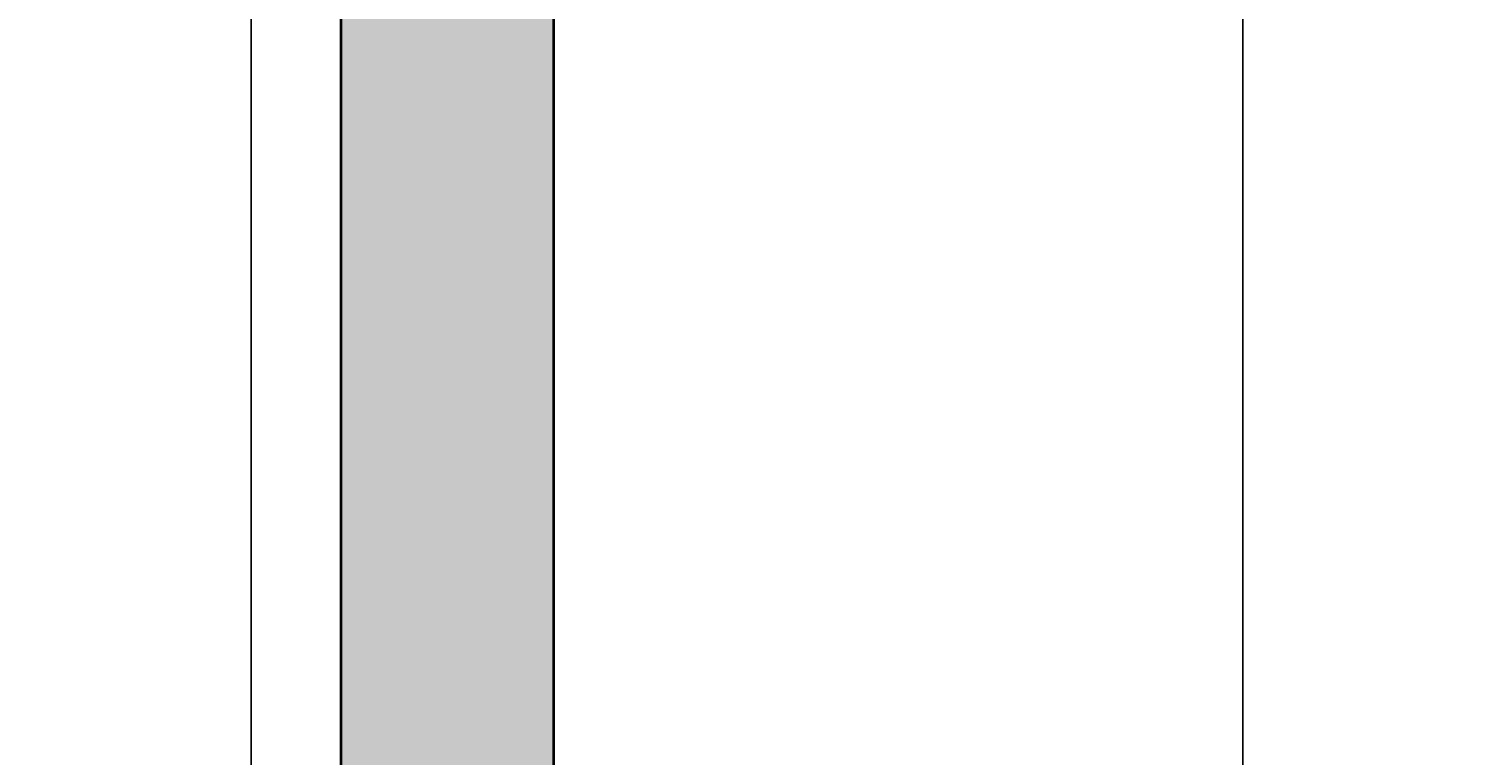
# Model space of a CAD drawing. Units: inches. Extents: x 1998 to 2588, y 1139 to 1977.
# Tile 131 of 134: x 2489 to 2550, y 1667 to 1698. Entities that reach past the tile are written whole.
import ezdxf

# ---------------------------------------------------------------- set-up
doc = ezdxf.new("R2010")
doc.units = ezdxf.units.IN
for name, color, linetype, lineweight in [('A-ANNO-DIMS', 2, 'Continuous', 18), ('A-WALL-PATT', 252, 'Continuous', 13), ('WALL', 200, 'Continuous', 35)]:
    doc.layers.add(name, color=color, linetype=linetype, lineweight=lineweight)
doc.styles.get("Standard").update_dxf_attribs({"font": 'arial.ttf'})
doc.dimstyles.get("Standard").update_dxf_attribs({"dimtxt": 0.18, "dimasz": 0.18, "dimexe": 0.18, "dimexo": 0.0625, "dimgap": 0.09, "dimtad": 0, "dimtih": 1, "dimtoh": 1, "dimdec": 4, "dimzin": 0, "dimdsep": 46, "dimtxsty": 'Standard', "dimcen": 0.09, "dimadec": 0, "dimazin": 0, "dimtfac": 1, "dimtdec": 4, "dimtofl": 0, "dimtmove": 0, "dimatfit": 3, "dimfxl": 1, "dimtolj": 1, "dimtzin": 0, "dimarcsym": 0})

# ---------------------------------------------------------------- blocks, each defined once
blk = doc.blocks.new('*D24')
at = {"layer": 'A-ANNO-DIMS', "color": 0, "lineweight": -2, "transparency": 16777216}
for p, q in [((2398.535, 1911.232), (2588.309, 1911.232)), ((2588.129, 1911.052), (2588.129, 1570.164)), ((2588.129, 1228.912), (2588.129, 1569.8)), ((2527.535, 1228.732), (2588.309, 1228.732))]:
    blk.add_line(p, q, dxfattribs=at)
at = {"layer": 'A-ANNO-DIMS', "color": 0, "transparency": 16777216}
for points in [[(2588.099, 1911.052), (2588.159, 1911.052), (2588.129, 1911.232)], [(2588.099, 1228.912), (2588.159, 1228.912), (2588.129, 1228.732)]]:
    blk.add_solid(points, dxfattribs=at)
at = {"layer": 'Defpoints', "color": 0, "transparency": 16777216}
for p in [(2398.473, 1911.232), (2588.129, 1911.232), (2527.473, 1228.732)]:
    blk.add_point(p, dxfattribs=at)
at = {"layer": 'A-ANNO-DIMS', "color": 0, "transparency": 16777216, "insert": (2588.129, 1569.982), "char_height": 0.18, "attachment_point": 5}
blk.add_mtext('\\A1;682.5', dxfattribs=at)
blk = doc.blocks.new('*D31')
at = {"layer": 'A-ANNO-DIMS', "color": 0, "lineweight": -2, "transparency": 16777216}
for p, q in [((2498.179, 1636.795), (2498.179, 1977.362)), ((2498.359, 1977.182), (2518.957, 1977.182)), ((2539.999, 1977.182), (2519.4, 1977.182)), ((2540.179, 1636.795), (2540.179, 1977.362))]:
    blk.add_line(p, q, dxfattribs=at)
at = {"layer": 'A-ANNO-DIMS', "color": 0, "transparency": 16777216}
for points in [[(2498.359, 1977.212), (2498.359, 1977.152), (2498.179, 1977.182)], [(2539.999, 1977.212), (2539.999, 1977.152), (2540.179, 1977.182)]]:
    blk.add_solid(points, dxfattribs=at)
at = {"layer": 'Defpoints', "color": 0, "transparency": 16777216}
for p in [(2540.179, 1977.182), (2498.179, 1636.732), (2540.179, 1636.732)]:
    blk.add_point(p, dxfattribs=at)
at = {"layer": 'A-ANNO-DIMS', "color": 0, "transparency": 16777216, "insert": (2519.179, 1977.182), "char_height": 0.18, "attachment_point": 5}
blk.add_mtext('\\A1;42', dxfattribs=at)

msp = doc.modelspace()

# ---------------------------------------------------------------- hatches: boundary and pattern name
at = {"layer": 'A-WALL-PATT'}
h = msp.add_hatch(color=256, dxfattribs=at)
h.dxf.hatch_style = 1
h.paths.add_polyline_path([(2527.4729, 1362.2324), (2510.9729, 1362.2324), (2510.9729, 1357.7324), (2518.4729, 1357.7324), (2518.4729, 1237.7324), (2503.1458, 1237.7324), (2503.1458, 1228.7324), (2527.4729, 1228.7324)])
h.paths.add_polyline_path([(2490.5682, 1362.2324), (2398.4729, 1362.2324), (2398.4729, 1357.7324), (2490.5682, 1357.7324)])
h.paths.add_polyline_path([(2224.9729, 1264.7324), (2222.9729, 1264.7324), (2222.9729, 1232.4125), (2341.4729, 1232.4125), (2341.4729, 1234.4125), (2224.9729, 1234.4125)])
h.paths.add_polyline_path([(2334.5332, 1273.7324), (2264.7638, 1273.7324), (2264.7638, 1269.5611, -0.043659), (2264.3413, 1264.7324), (2334.5332, 1264.7324)])
h.paths.add_polyline_path([(2236.9551, 1273.7324), (2234.4125, 1273.7324), (2234.4125, 1264.7324), (2236.9551, 1264.7324), (2236.9551, 1269.5611)])
h.paths.add_polyline_path([(2222.9729, 1293.2324), (2096.9729, 1293.2324), (2096.9729, 1345.0966), (2087.9729, 1345.0966), (2087.9729, 1284.2324), (2222.9729, 1284.2324), (2222.9729, 1285.137)])
h.paths.add_polyline_path([(2096.9729, 1458.7927), (2087.9729, 1458.7927), (2087.9729, 1417.7324), (2087.9729, 1413.2324), (2096.9729, 1413.2324), (2096.9729, 1417.7324)])
h.paths.add_polyline_path([(2096.9729, 1413.2324), (2087.9729, 1413.2324), (2087.9729, 1365.5012), (2096.9729, 1365.5012), (2096.9729, 1369.3358)])
h.paths.add_polyline_path([(2186.2943, 1417.7324), (2138.6074, 1417.7324), (2096.9729, 1417.7324), (2096.9729, 1413.2324), (2138.6074, 1413.2324), (2186.2943, 1413.2324)])
h.paths.add_polyline_path([(2181.4729, 1465.7324), (2176.9729, 1465.7324), (2176.9729, 1451.6434), (2181.4729, 1451.6434)])
h.paths.add_polyline_path([(2181.4729, 1422.1664), (2176.9729, 1422.1664), (2176.9729, 1417.7324), (2181.4729, 1417.7324)])
h.paths.add_polyline_path([(2063.9729, 1465.7324), (2087.9729, 1465.7324), (2087.9729, 1470.2324), (2059.4729, 1470.2324), (2059.4729, 1413.2324), (2087.9729, 1413.2324), (2087.9729, 1417.7324), (2063.9729, 1417.7324)])
h.paths.add_polyline_path([(2181.4729, 1755.2324), (2176.9729, 1755.2324), (2176.9729, 1748.6798), (2177.0513, 1748.6798), (2181.4729, 1748.6798)])
h.paths.add_polyline_path([(2227.4729, 1707.2324), (2220.4647, 1707.2324), (2220.4647, 1702.7324), (2222.9729, 1702.7324), (2222.9729, 1604.637), (2227.4729, 1604.637)])
h.paths.add_polyline_path([(2114.9729, 1702.7324), (2105.9729, 1702.7324), (2105.9729, 1628.4781, -0.0318759), (2110.1012, 1628.7416), (2114.9729, 1628.7416)])
h.paths.add_polyline_path([(2345.9729, 1739.3278), (2341.4729, 1739.3278), (2341.4729, 1647.5211), (2345.9729, 1647.5211)])
h.paths.add_polyline_path([(2350.6273, 1641.2324), (2345.9729, 1641.2324), (2345.9729, 1636.7324), (2350.6273, 1636.7324), (2350.6273, 1639.8729)])
h.paths.add_polyline_path([(2501.9729, 1641.2324), (2407.9729, 1641.2324), (2392.5005, 1641.2324), (2392.5005, 1639.8729), (2392.5005, 1636.7324), (2501.9729, 1636.7324)])
h.paths.add_polyline_path([(2510.9729, 1755.2324), (2501.9729, 1755.2324), (2501.9729, 1641.2324), (2510.9729, 1641.2324)])
h.paths.add_polyline_path([(2549.1786, 1641.2324), (2522.3775, 1641.2324), (2522.3775, 1636.7324), (2540.1786, 1636.7324), (2540.1786, 1480.7324), (2522.3775, 1480.7324), (2522.3775, 1476.2324), (2549.1786, 1476.2324)])
h.paths.add_polyline_path([(2498.1786, 1594.7324), (2407.9729, 1594.7324), (2407.9729, 1585.7324), (2416.9729, 1585.7324), (2489.1786, 1585.7324), (2489.1786, 1531.7324), (2416.9729, 1531.7324), (2407.9729, 1531.7324), (2407.9729, 1522.7324), (2498.1786, 1522.7324)])
h.paths.add_polyline_path([(2351.6437, 1480.7324), (2345.9729, 1480.7324), (2345.9729, 1476.2324), (2351.6437, 1476.2324), (2351.6437, 1477.5919)])
h.paths.add_polyline_path([(2501.9729, 1480.7324), (2498.1786, 1480.7324), (2407.9729, 1480.7324), (2393.5168, 1480.7324), (2393.5168, 1477.5919), (2393.5168, 1476.2324), (2501.9729, 1476.2324)])

# ---------------------------------------------------------------- linework, layer by layer
at = {"layer": 'WALL'}
for p, q in [((2501.9729, 1755.2324), (2501.9729, 1641.2324)), ((2510.9729, 1755.2324), (2510.9729, 1641.2324))]:
    msp.add_line(p, q, dxfattribs=at)

# ---------------------------------------------------------------- dimensions: what is measured, and where the dimension line sits
at = {"layer": 'A-ANNO-DIMS'}
dim = msp.add_linear_dim(base=(2540.1786, 1977.1824), p1=(2498.1786, 1636.7324), p2=(2540.1786, 1636.7324), dimstyle='Standard', override={"dimdec": 0, "dimlfac": 1, "dimrnd": 0, "dimzin": 0, "dimdsep": 46, "dimlunit": 2}, dxfattribs=at)
dim.commit()
dim.dimension.update_dxf_attribs({"geometry": '*D31', "text_midpoint": (2519.1786, 1977.1824)})
dim = msp.add_linear_dim(base=(2588.1286, 1911.2324), p1=(2527.4729, 1228.7324), p2=(2398.4729, 1911.2324), angle=90, dimstyle='Standard', override={"dimdec": 1, "dimlfac": 1, "dimrnd": 0, "dimzin": 0, "dimdsep": 46, "dimlunit": 2}, dxfattribs=at)
dim.commit()
dim.dimension.update_dxf_attribs({"geometry": '*D24', "text_midpoint": (2588.1286, 1569.9824)})

doc.saveas('drawing.dxf')
